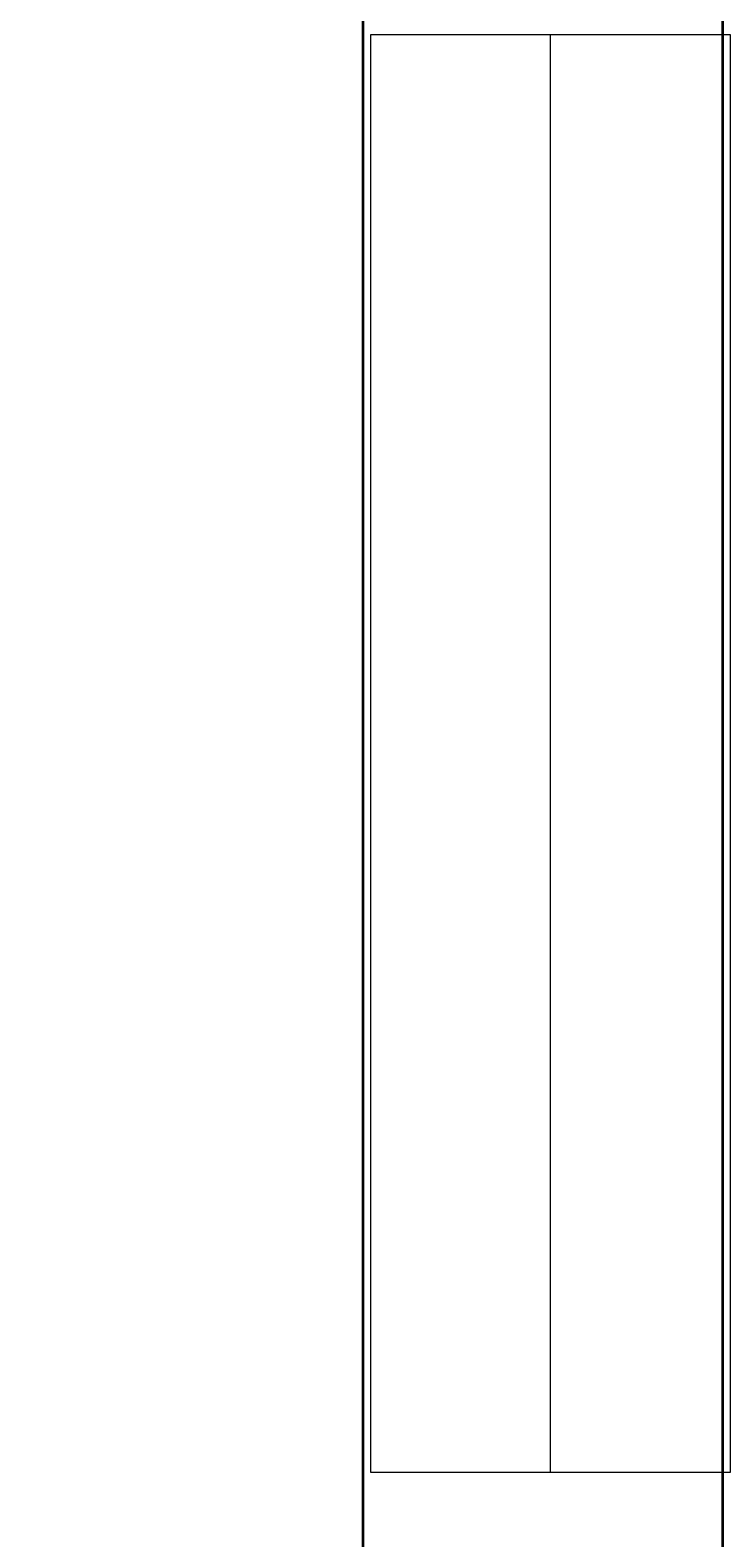
# Model space of a CAD drawing. Units: millimetres. Extents: x 27017497 to 27018854, y 7058029 to 7059154.
# Tile 11 of 91: x 27017605 to 27017623, y 7058200 to 7058238. Entities that reach past the tile are written whole.
import ezdxf

# ---------------------------------------------------------------- set-up
doc = ezdxf.new("R2010")
doc.units = ezdxf.units.MM
for name, color, linetype, lineweight in [('A-ANNO-DIMS', 2, 'Continuous', 18), ('A-GLAZ', 4, 'Continuous', 18), ('A-WALL', 7, 'Continuous', 35)]:
    doc.layers.add(name, color=color, linetype=linetype, lineweight=lineweight)
doc.styles.get("Standard").update_dxf_attribs({"font": 'arial.ttf'})
doc.dimstyles.get("Standard").update_dxf_attribs({"dimtxt": 0.18, "dimasz": 0.18, "dimexe": 0.18, "dimexo": 0.0625, "dimgap": 0.09, "dimtad": 0, "dimtih": 1, "dimtoh": 1, "dimdec": 4, "dimzin": 0, "dimdsep": 46, "dimtxsty": 'Standard', "dimcen": 0.09, "dimadec": 0, "dimazin": 0, "dimtfac": 1, "dimtdec": 4, "dimtofl": 0, "dimtmove": 0, "dimatfit": 3, "dimfxl": 1, "dimtolj": 1, "dimtzin": 0, "dimarcsym": 0})

# ---------------------------------------------------------------- blocks, each defined once
blk = doc.blocks.new('WINDOW-SINGLE-LIGHT')
blk.add_lwpolyline([(36, 4.5), (36, 0), (0, 0), (0, 9), (36, 9), (36, 4.5), (0, 4.5)])
blk = doc.blocks.new('*D47')
at = {"layer": 'A-ANNO-DIMS', "color": 0, "lineweight": -2, "transparency": 16777216}
for p, q in [((27017561.166, 7058294.35), (27017561.166, 7058028.6)), ((27018790.606, 7058294.35), (27018790.606, 7058028.6)), ((27017561.346, 7058028.78), (27018175.431, 7058028.78)), ((27018790.426, 7058028.78), (27018176.341, 7058028.78))]:
    blk.add_line(p, q, dxfattribs=at)
at = {"layer": 'A-ANNO-DIMS', "color": 0, "transparency": 16777216}
for points in [[(27017561.346, 7058028.81), (27017561.346, 7058028.75), (27017561.166, 7058028.78)], [(27018790.426, 7058028.81), (27018790.426, 7058028.75), (27018790.606, 7058028.78)]]:
    blk.add_solid(points, dxfattribs=at)
at = {"layer": 'Defpoints', "color": 0, "transparency": 16777216}
for p in [(27017561.166, 7058294.412), (27018790.606, 7058294.412), (27018790.606, 7058028.78)]:
    blk.add_point(p, dxfattribs=at)
at = {"layer": 'A-ANNO-DIMS', "color": 0, "transparency": 16777216, "insert": (27018175.886, 7058028.78), "char_height": 0.18, "attachment_point": 5}
blk.add_mtext('\\A1;1229.4', dxfattribs=at)
blk = doc.blocks.new('*D48')
at = {"layer": 'A-ANNO-DIMS', "color": 0, "lineweight": -2, "transparency": 16777216}
for p, q in [((27018463.498, 7058622.912), (27017497.536, 7058622.912)), ((27017497.716, 7058622.732), (27017497.716, 7058357.753)), ((27017497.716, 7058092.41), (27017497.716, 7058357.389)), ((27018555.129, 7058092.23), (27017497.536, 7058092.23))]:
    blk.add_line(p, q, dxfattribs=at)
at = {"layer": 'A-ANNO-DIMS', "color": 0, "transparency": 16777216}
for points in [[(27017497.686, 7058622.732), (27017497.746, 7058622.732), (27017497.716, 7058622.912)], [(27017497.686, 7058092.41), (27017497.746, 7058092.41), (27017497.716, 7058092.23)]]:
    blk.add_solid(points, dxfattribs=at)
at = {"layer": 'Defpoints', "color": 0, "transparency": 16777216}
for p in [(27018463.561, 7058622.912), (27017497.716, 7058092.23), (27018555.192, 7058092.23)]:
    blk.add_point(p, dxfattribs=at)
at = {"layer": 'A-ANNO-DIMS', "color": 0, "transparency": 16777216, "insert": (27017497.716, 7058357.571), "char_height": 0.18, "attachment_point": 5}
blk.add_mtext('\\A1;530.7', dxfattribs=at)

msp = doc.modelspace()

# ---------------------------------------------------------------- linework, layer by layer
at = {"layer": 'A-WALL'}
for p, q in [((27017613.666, 7058294.412), (27017613.666, 7058132.912)), ((27017622.666, 7058294.412), (27017622.666, 7058141.912))]:
    msp.add_line(p, q, dxfattribs=at)

# ---------------------------------------------------------------- block references
at = {"layer": 'A-GLAZ', "rotation": 270}
msp.add_blockref('WINDOW-SINGLE-LIGHT', (27017613.865, 7058237.7), dxfattribs=at)

# ---------------------------------------------------------------- dimensions: what is measured, and where the dimension line sits
at = {"layer": 'A-ANNO-DIMS'}
dim = msp.add_linear_dim(base=(27017497.716, 7058092.23), p1=(27018463.561, 7058622.912), p2=(27018555.192, 7058092.23), angle=90, dimstyle='Standard', override={"dimdec": 1, "dimlfac": 1, "dimrnd": 0, "dimzin": 0, "dimdsep": 46, "dimlunit": 2}, dxfattribs=at)
dim.commit()
dim.dimension.update_dxf_attribs({"geometry": '*D48', "text_midpoint": (27017497.716, 7058357.571)})
dim = msp.add_linear_dim(base=(27018790.606, 7058028.78), p1=(27017561.166, 7058294.412), p2=(27018790.606, 7058294.412), dimstyle='Standard', override={"dimdec": 1, "dimlfac": 1, "dimrnd": 0, "dimzin": 0, "dimdsep": 46, "dimlunit": 2}, dxfattribs=at)
dim.commit()
dim.dimension.update_dxf_attribs({"geometry": '*D47', "text_midpoint": (27018175.886, 7058028.78)})

doc.saveas('drawing.dxf')
